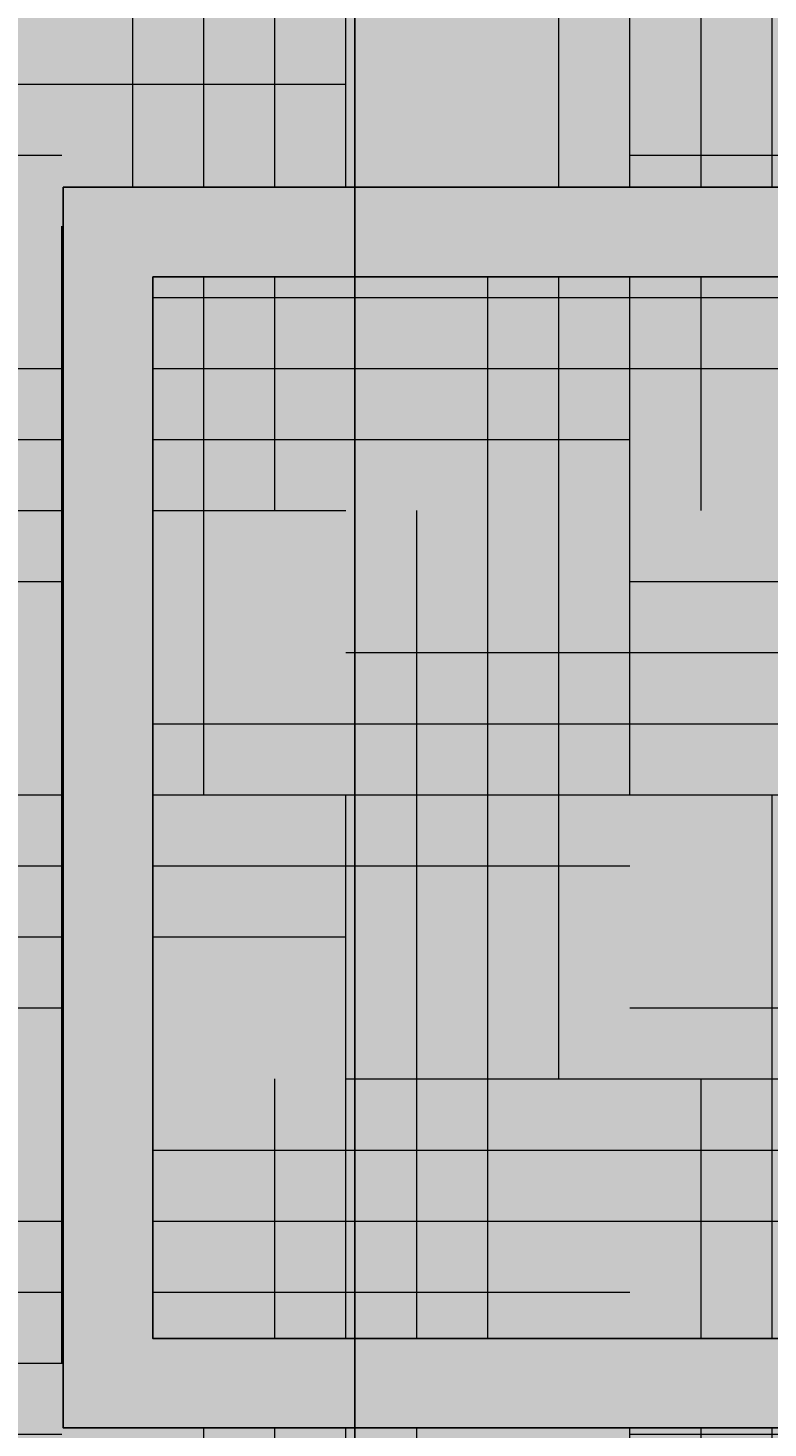
# Model space of a CAD drawing. Units: feet. Extents: x 2695 to 2912, y 795 to 1139.
# Tile 11 of 83: x 2723 to 2740, y 875 to 906. Entities that reach past the tile are written whole.
import ezdxf

# ---------------------------------------------------------------- set-up
doc = ezdxf.new("R2010")
doc.units = ezdxf.units.FT
for name, color, linetype, lineweight in [('A-ANNO-DIMS', 2, 'Continuous', 18), ('A-ELEV-PATT', 252, 'Continuous', 13), ('A-GLAZ', 4, 'Continuous', 25), ('A-GLAZ-PATT', 254, 'Continuous', 13)]:
    doc.layers.add(name, color=color, linetype=linetype, lineweight=lineweight)
doc.styles.get("Standard").update_dxf_attribs({"font": 'arial.ttf'})
doc.dimstyles.get("Standard").update_dxf_attribs({"dimtxt": 0.18, "dimasz": 0.18, "dimexe": 0.18, "dimexo": 0.0625, "dimgap": 0.09, "dimtad": 0, "dimtih": 1, "dimtoh": 1, "dimdec": 1, "dimzin": 0, "dimdsep": 46, "dimlunit": 3, "dimtxsty": 'Standard', "dimcen": 0.09, "dimadec": 0, "dimazin": 0, "dimtfac": 1, "dimtdec": 1, "dimtofl": 0, "dimtmove": 0, "dimatfit": 3, "dimfxl": 1, "dimtolj": 1, "dimtzin": 0, "dimarcsym": 0})

# ---------------------------------------------------------------- blocks, each defined once
blk = doc.blocks.new('*D23')
at = {"layer": 'A-ANNO-DIMS', "color": 0, "lineweight": -2, "transparency": 16777216}
for p, q in [((2715.885, 936.868), (2715.885, 794.976)), ((2730.708, 936.868), (2730.708, 794.976)), ((2716.065, 795.156), (2722.842, 795.156)), ((2730.528, 795.156), (2723.752, 795.156))]:
    blk.add_line(p, q, dxfattribs=at)
at = {"layer": 'A-ANNO-DIMS', "color": 0, "transparency": 16777216}
for points in [[(2716.065, 795.186), (2716.065, 795.126), (2715.885, 795.156)], [(2730.528, 795.186), (2730.528, 795.126), (2730.708, 795.156)]]:
    blk.add_solid(points, dxfattribs=at)
at = {"layer": 'Defpoints', "color": 0, "transparency": 16777216}
for p in [(2715.885, 936.931), (2730.708, 936.931), (2730.708, 795.156)]:
    blk.add_point(p, dxfattribs=at)
at = {"layer": 'A-ANNO-DIMS', "color": 0, "transparency": 16777216, "insert": (2723.297, 795.156), "char_height": 0.18, "attachment_point": 5}
blk.add_mtext('\\A1;14.823', dxfattribs=at)
blk = doc.blocks.new('*D24')
at = {"layer": 'A-ANNO-DIMS', "color": 0, "lineweight": -2, "transparency": 16777216}
for p, q in [((2730.708, 936.868), (2730.708, 794.976)), ((2755.112, 936.868), (2755.112, 794.976)), ((2730.888, 795.156), (2742.446, 795.156)), ((2754.932, 795.156), (2743.375, 795.156))]:
    blk.add_line(p, q, dxfattribs=at)
at = {"layer": 'A-ANNO-DIMS', "color": 0, "transparency": 16777216}
for points in [[(2730.888, 795.186), (2730.888, 795.126), (2730.708, 795.156)], [(2754.932, 795.186), (2754.932, 795.126), (2755.112, 795.156)]]:
    blk.add_solid(points, dxfattribs=at)
at = {"layer": 'Defpoints', "color": 0, "transparency": 16777216}
for p in [(2730.708, 936.931), (2755.112, 936.931), (2755.112, 795.156)]:
    blk.add_point(p, dxfattribs=at)
at = {"layer": 'A-ANNO-DIMS', "color": 0, "transparency": 16777216, "insert": (2742.91, 795.156), "char_height": 0.18, "attachment_point": 5}
blk.add_mtext('\\A1;24.404', dxfattribs=at)

msp = doc.modelspace()

# ---------------------------------------------------------------- hatches: boundary and pattern name
at = {"layer": 'A-ELEV-PATT'}
h = msp.add_hatch(color=256, dxfattribs=at)
h.set_gradient(color2=(0, 0, 0), tint=1)
h.paths.add_polyline_path([(2772.5216, 971.9673), (2770.6361, 971.9673), (2770.6361, 970.7156), (2772.5216, 970.7156)])
h.paths.add_polyline_path([(2773.2702, 971.9673), (2772.5216, 971.9673), (2772.5216, 970.7156), (2773.2702, 970.7156)])
h.paths.add_polyline_path([(2778.0341, 971.9673), (2773.2702, 971.9673), (2773.2702, 970.7156), (2778.0341, 970.7156)])
h.paths.add_polyline_path([(2780.0341, 971.9673), (2778.0341, 971.9673), (2778.0341, 970.7156), (2780.0341, 970.7156)])
h.paths.add_polyline_path([(2841.575, 971.9673), (2780.0341, 971.9673), (2780.0341, 970.7156), (2841.575, 970.7156)])
h.paths.add_polyline_path([(2843.575, 971.9673), (2841.575, 971.9673), (2841.575, 970.7156), (2843.575, 970.7156)])
h.paths.add_polyline_path([(2888.1882, 971.9673), (2843.575, 971.9673), (2843.575, 970.7156), (2888.1882, 970.7156)])
h.paths.add_polyline_path([(2888.9368, 971.9673), (2888.1882, 971.9673), (2888.1882, 970.7156), (2888.9368, 970.7156)], flags=17)
h.paths.add_polyline_path([(2890.6361, 971.9673), (2888.9368, 971.9673), (2888.9368, 970.7156), (2890.6361, 970.7156)])
h.paths.add_polyline_path([(2888.9368, 971.9673), (2888.1882, 971.9673), (2888.1882, 964.8267), (2888.9368, 964.8267)])
h.paths.add_polyline_path([(2888.9368, 964.8267), (2888.1882, 964.8267), (2888.1882, 964.1328), (2888.9368, 964.1328)])
h.paths.add_polyline_path([(2890.6361, 964.8267), (2888.9368, 964.8267), (2888.9368, 964.1328), (2890.6361, 964.1328)])
h.paths.add_polyline_path([(2888.1882, 964.8267), (2770.6361, 964.8267), (2770.6361, 964.1328), (2888.1882, 964.1328)])
h.paths.add_polyline_path([(2888.9368, 964.1328), (2888.1882, 964.1328), (2888.1882, 936.9306), (2888.9368, 936.9306)])
h.paths.add_polyline_path([(2890.6361, 956.614), (2888.9368, 956.614), (2888.9368, 955.9202), (2890.6361, 955.9202)])
h.paths.add_polyline_path([(2888.1882, 956.614), (2770.6361, 956.614), (2770.6361, 955.9202), (2888.1882, 955.9202)])
h.paths.add_polyline_path([(2890.6361, 949.2892), (2888.9368, 949.2892), (2888.9368, 948.5954), (2890.6361, 948.5954)])
h.paths.add_polyline_path([(2888.1882, 949.2892), (2770.6361, 949.2892), (2770.6361, 948.5954), (2888.1882, 948.5954)])
h.paths.add_polyline_path([(2890.6361, 941.3507), (2888.9368, 941.3507), (2888.9368, 940.6569), (2890.6361, 940.6569)])
h.paths.add_polyline_path([(2888.1882, 941.3507), (2770.6361, 941.3507), (2770.6361, 940.6569), (2888.1882, 940.6569)])
h.paths.add_polyline_path([(2773.2702, 970.7156), (2772.5216, 970.7156), (2772.5216, 964.8267), (2773.2702, 964.8267)])
h.paths.add_polyline_path([(2773.2702, 964.1328), (2772.5216, 964.1328), (2772.5216, 956.614), (2773.2702, 956.614)])
h.paths.add_polyline_path([(2773.2702, 955.9202), (2772.5216, 955.9202), (2772.5216, 936.9306), (2773.2702, 936.9306)])
h.paths.add_polyline_path([(2810.7893, 970.7156), (2810.0407, 970.7156), (2810.0407, 964.8267), (2810.7893, 964.8267)], flags=17)
h.paths.add_polyline_path([(2810.7893, 964.1328), (2810.0407, 964.1328), (2810.0407, 956.614), (2810.7893, 956.614)], flags=17)
h.paths.add_polyline_path([(2810.7893, 955.9202), (2810.0407, 955.9202), (2810.0407, 949.2892), (2810.7893, 949.2892)], flags=17)
h.paths.add_polyline_path([(2810.7893, 971.9673), (2810.0407, 971.9673), (2810.0407, 941.3507), (2810.7893, 941.3507)])
h.paths.add_polyline_path([(2810.7893, 940.6569), (2810.0407, 940.6569), (2810.0407, 936.9306), (2810.7893, 936.9306)])
h.paths.add_polyline_path([(2780.0341, 1018.8235), (2841.575, 1018.8235), (2841.575, 971.9673), (2843.575, 971.9673), (2843.575, 1020.8235), (2778.0341, 1020.8235), (2778.0341, 971.9673), (2780.0341, 971.9673)])
h.paths.add_polyline_path([(2780.0341, 970.7156), (2778.0341, 970.7156), (2778.0341, 964.8267), (2780.0341, 964.8267)])
h.paths.add_polyline_path([(2780.0341, 964.1328), (2778.0341, 964.1328), (2778.0341, 956.614), (2780.0341, 956.614)])
h.paths.add_polyline_path([(2780.0341, 955.9202), (2778.0341, 955.9202), (2778.0341, 949.2892), (2780.0341, 949.2892)])
h.paths.add_polyline_path([(2780.0341, 948.5954), (2778.0341, 948.5954), (2778.0341, 941.3507), (2780.0341, 941.3507)])
h.paths.add_polyline_path([(2780.0341, 940.6569), (2778.0341, 940.6569), (2778.0341, 936.9306), (2780.0341, 936.9306)])
h.paths.add_polyline_path([(2843.575, 940.6569), (2841.575, 940.6569), (2841.575, 936.9306), (2843.575, 936.9306)])
h.paths.add_polyline_path([(2843.575, 948.5954), (2841.575, 948.5954), (2841.575, 941.3507), (2843.575, 941.3507)])
h.paths.add_polyline_path([(2843.575, 970.7156), (2841.575, 970.7156), (2841.575, 964.8267), (2843.575, 964.8267)])
h.paths.add_polyline_path([(2843.575, 964.1328), (2841.575, 964.1328), (2841.575, 956.614), (2843.575, 956.614)])
h.paths.add_polyline_path([(2843.575, 955.9202), (2841.575, 955.9202), (2841.575, 949.2892), (2843.575, 949.2892)])
h.paths.add_polyline_path([(2805.0538, 874.1057), (2803.9681, 874.1057), (2803.9681, 846.2857), (2805.0538, 846.2857)])
h.paths.add_polyline_path([(2758.1515, 902.577), (2724.1893, 902.577), (2724.1893, 874.8571), (2758.1515, 874.8571)])
h.paths.add_polyline_path([(2726.1893, 900.577), (2756.1515, 900.577), (2756.1515, 876.8571), (2726.1893, 876.8571)], flags=16)
h.paths.add_polyline_path([(2740.7302, 900.577), (2741.6105, 900.577), (2741.6105, 876.8571), (2740.7302, 876.8571)], flags=0)
h = msp.add_hatch(color=256, dxfattribs=at)
h.set_gradient(color1=(255, 255, 255))
h.paths.add_polyline_path([(2770.6361, 924.3105), (2716.5358, 924.3105), (2716.5358, 810.9306), (2770.6361, 810.9306)])
h.paths.add_polyline_path([(2758.1515, 902.577), (2758.1515, 874.8571), (2724.1893, 874.8571), (2724.1893, 902.577)], flags=16)
h.paths.add_polyline_path([(2756.1515, 900.577), (2756.1515, 876.8571), (2726.1893, 876.8571), (2726.1893, 900.577)], flags=0)
h.paths.add_polyline_path([(2740.7302, 900.577), (2741.6105, 900.577), (2741.6105, 876.8571), (2740.7302, 876.8571)], flags=0)
h = msp.add_hatch(dxfattribs=at)
h.set_pattern_fill('HOUND', color=256, style=0)
h.paths.add_polyline_path([(2770.6361, 924.3105), (2716.5358, 924.3105), (2716.5358, 810.9306), (2770.6361, 810.9306)])
h.paths.add_polyline_path([(2724.1893, 874.8571), (2724.1893, 902.577), (2758.1515, 902.577), (2758.1515, 874.8571)], flags=16)
h.paths.add_polyline_path([(2756.1515, 876.8571), (2726.1893, 876.8571), (2726.1893, 900.577), (2756.1515, 900.577)], flags=0)
h.paths.add_polyline_path([(2741.6105, 876.8571), (2740.7302, 876.8571), (2740.7302, 900.577), (2741.6105, 900.577)], flags=0)
at = {"layer": 'A-GLAZ-PATT'}
h = msp.add_hatch(color=256, dxfattribs=at)
h.set_gradient(color1=(153, 185, 219), color2=(153, 185, 219))
h.paths.add_polyline_path([(2740.7302, 900.577), (2726.1893, 900.577), (2726.1893, 876.8571), (2740.7302, 876.8571)])
h.paths.add_polyline_path([(2756.1515, 900.577), (2741.6105, 900.577), (2741.6105, 876.8571), (2756.1515, 876.8571)])
h = msp.add_hatch(color=256, dxfattribs=at)
h.set_gradient(color1=(153, 185, 219), color2=(153, 185, 219))
h.paths.add_polyline_path([(2740.7302, 900.577), (2726.1893, 900.577), (2726.1893, 876.8571), (2740.7302, 876.8571)])
h.paths.add_polyline_path([(2756.1515, 900.577), (2741.6105, 900.577), (2741.6105, 876.8571), (2756.1515, 876.8571)])

# ---------------------------------------------------------------- linework, layer by layer
at = {"layer": 'A-GLAZ'}
for p, q in [((2724.1893, 902.577), (2758.1515, 902.577)), ((2724.1893, 874.8571), (2724.1893, 902.577)), ((2758.1515, 874.8571), (2724.1893, 874.8571))]:
    msp.add_line(p, q, dxfattribs=at)
for points in [[(2724.1893, 902.577), (2758.1515, 902.577), (2758.1515, 874.8571), (2724.1893, 874.8571)], [(2726.1893, 900.577), (2756.1515, 900.577), (2756.1515, 876.8571), (2726.1893, 876.8571)], [(2726.1893, 900.577), (2756.1515, 900.577), (2756.1515, 876.8571), (2726.1893, 876.8571)]]:
    msp.add_lwpolyline(points, close=True, dxfattribs=at)

# ---------------------------------------------------------------- dimensions: what is measured, and where the dimension line sits
at = {"layer": 'A-ANNO-DIMS'}
for base, p1, p2, picture, middle in [((2730.7081, 795.1556), (2715.8852, 936.9306), (2730.7081, 936.9306), '*D23', (2723.2967, 795.1556)), ((2755.1125, 795.1556), (2730.7081, 936.9306), (2755.1125, 936.9306), '*D24', (2742.9103, 795.1556))]:
    dim = msp.add_linear_dim(base=base, p1=p1, p2=p2, dimstyle='Standard', override={"dimdec": 3, "dimlfac": 1, "dimrnd": 0, "dimzin": 0, "dimdsep": 46, "dimlunit": 2}, dxfattribs=at)
    dim.commit()
    dim.dimension.update_dxf_attribs({"geometry": picture, "text_midpoint": middle})

doc.saveas('drawing.dxf')
